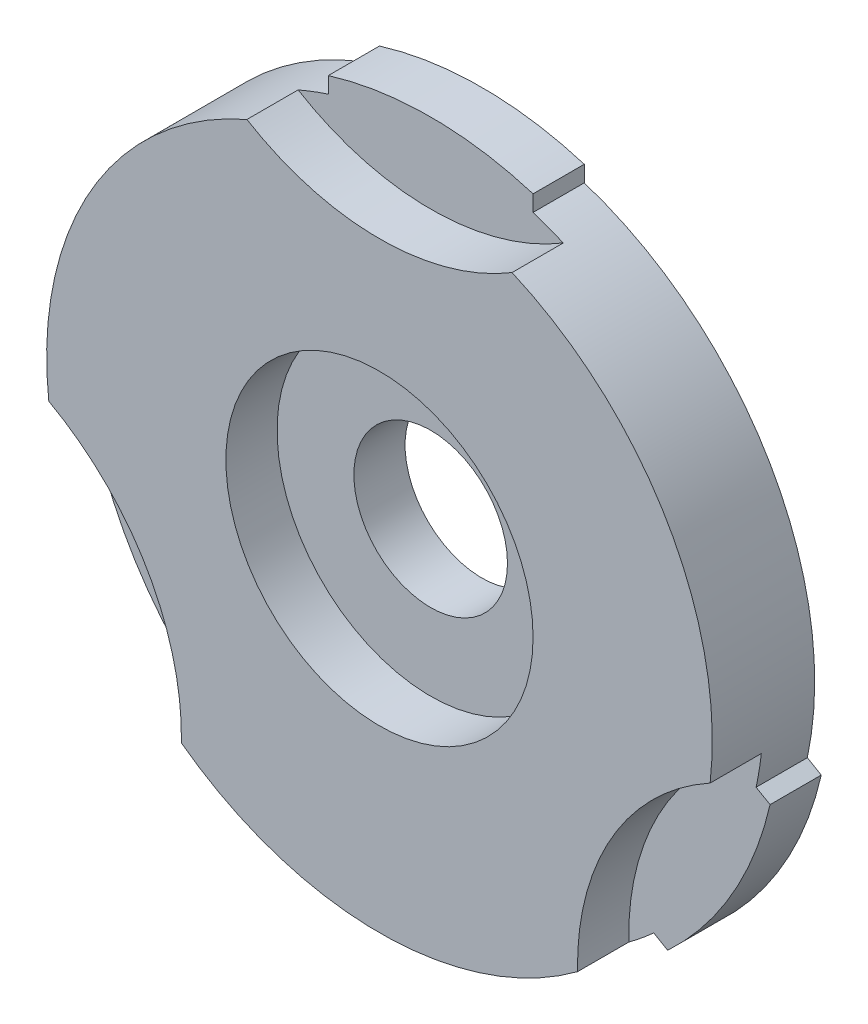
ISO-10303-21;
HEADER;
FILE_DESCRIPTION(('STEP AP214'),'2;1');
FILE_NAME('part.step','',(''),(''),'','','');
FILE_SCHEMA(('AUTOMOTIVE_DESIGN { 1 0 10303 214 1 1 1 1 }'));
ENDSEC;
DATA;
#1=APPLICATION_CONTEXT('core data for automotive mechanical design processes');
#2=APPLICATION_PROTOCOL_DEFINITION('international standard','automotive_design',2000,#1);
#3=PRODUCT_CONTEXT('',#1,'mechanical');
#4=PRODUCT('Part','Part','',(#3));
#5=PRODUCT_RELATED_PRODUCT_CATEGORY('part','',(#4));
#6=PRODUCT_DEFINITION_FORMATION('','',#4);
#7=PRODUCT_DEFINITION_CONTEXT('part definition',#1,'design');
#8=PRODUCT_DEFINITION('design','',#6,#7);
#9=PRODUCT_DEFINITION_SHAPE('','',#8);
#10=(LENGTH_UNIT() NAMED_UNIT(*) SI_UNIT(.MILLI.,.METRE.));
#11=(NAMED_UNIT(*) PLANE_ANGLE_UNIT() SI_UNIT($,.RADIAN.));
#12=(NAMED_UNIT(*) SI_UNIT($,.STERADIAN.) SOLID_ANGLE_UNIT());
#13=UNCERTAINTY_MEASURE_WITH_UNIT(LENGTH_MEASURE(1.E-05),#10,'distance_accuracy_value','');
#14=(GEOMETRIC_REPRESENTATION_CONTEXT(3) GLOBAL_UNCERTAINTY_ASSIGNED_CONTEXT((#13)) GLOBAL_UNIT_ASSIGNED_CONTEXT((#10,
#11,#12)) REPRESENTATION_CONTEXT('',''));
#15=CARTESIAN_POINT('',(0.,0.,0.));
#16=DIRECTION('',(0.,0.,1.));
#17=DIRECTION('',(1.,0.,0.));
#18=AXIS2_PLACEMENT_3D('',#15,#16,#17);
#19=CARTESIAN_POINT('',(0.,0.,10.));
#20=DIRECTION('',(0.,0.,1.));
#21=DIRECTION('',(1.,0.,0.));
#22=AXIS2_PLACEMENT_3D('',#19,#20,#21);
#23=PLANE('',#22);
#24=CARTESIAN_POINT('',(0.,102.394299444478,10.));
#25=DIRECTION('',(0.,0.,-1.));
#26=DIRECTION('',(1.,0.,0.));
#27=AXIS2_PLACEMENT_3D('',#24,#25,#26);
#28=CIRCLE('',#27,50.);
#29=CARTESIAN_POINT('',(25.8920747012508,59.6204702066735,10.));
#30=VERTEX_POINT('',#29);
#31=CARTESIAN_POINT('',(-25.8920747012508,59.6204702066735,10.));
#32=VERTEX_POINT('',#31);
#33=EDGE_CURVE('E53',#30,#32,#28,.T.);
#34=ORIENTED_EDGE('',*,*,#33,.F.);
#35=CARTESIAN_POINT('',(0.,0.,10.));
#36=DIRECTION('',(0.,0.,1.));
#37=DIRECTION('',(1.,0.,0.));
#38=AXIS2_PLACEMENT_3D('',#35,#36,#37);
#39=CIRCLE('',#38,65.);
#40=CARTESIAN_POINT('',(20.,61.8465843842649,10.));
#41=VERTEX_POINT('',#40);
#42=EDGE_CURVE('E222',#30,#41,#39,.T.);
#43=ORIENTED_EDGE('',*,*,#42,.T.);
#44=DIRECTION('',(0.,1.,0.));
#45=VECTOR('',#44,1.);
#46=CARTESIAN_POINT('',(20.,61.8465843842649,10.));
#47=LINE('',#46,#45);
#48=CARTESIAN_POINT('',(20.0000000000001,64.9923072370939,10.));
#49=VERTEX_POINT('',#48);
#50=EDGE_CURVE('E224',#41,#49,#47,.T.);
#51=ORIENTED_EDGE('',*,*,#50,.T.);
#52=CARTESIAN_POINT('',(0.,0.,10.));
#53=DIRECTION('',(0.,0.,1.));
#54=DIRECTION('',(1.,0.,0.));
#55=AXIS2_PLACEMENT_3D('',#52,#53,#54);
#56=CIRCLE('',#55,68.000000000006);
#57=CARTESIAN_POINT('',(-20.,64.9923072370939,10.));
#58=VERTEX_POINT('',#57);
#59=EDGE_CURVE('E197',#49,#58,#56,.T.);
#60=ORIENTED_EDGE('',*,*,#59,.T.);
#61=DIRECTION('',(0.,-1.,0.));
#62=VECTOR('',#61,1.);
#63=CARTESIAN_POINT('',(-20.,61.8465843842649,10.));
#64=LINE('',#63,#62);
#65=CARTESIAN_POINT('',(-20.,61.8465843842649,10.));
#66=VERTEX_POINT('',#65);
#67=EDGE_CURVE('E199',#58,#66,#64,.T.);
#68=ORIENTED_EDGE('',*,*,#67,.T.);
#69=CARTESIAN_POINT('',(0.,0.,10.));
#70=DIRECTION('',(0.,0.,1.));
#71=DIRECTION('',(1.,0.,0.));
#72=AXIS2_PLACEMENT_3D('',#69,#70,#71);
#73=CIRCLE('',#72,65.);
#74=EDGE_CURVE('E204',#66,#32,#73,.T.);
#75=ORIENTED_EDGE('',*,*,#74,.T.);
#76=EDGE_LOOP('',(#34,#43,#51,#60,#68,#75));
#77=FACE_BOUND('',#76,.T.);
#78=ADVANCED_FACE('F39',(#77),#23,.T.);
#79=CARTESIAN_POINT('',(88.6760645216287,-51.1971497222389,10.));
#80=DIRECTION('',(0.,0.,-1.));
#81=DIRECTION('',(1.,0.,0.));
#82=AXIS2_PLACEMENT_3D('',#79,#80,#81);
#83=CIRCLE('',#82,49.9999999999992);
#84=CARTESIAN_POINT('',(38.686804433928,-52.2334295513037,10.));
#85=VERTEX_POINT('',#84);
#86=CARTESIAN_POINT('',(64.5788791351778,-7.38704065537017,10.));
#87=VERTEX_POINT('',#86);
#88=EDGE_CURVE('E183',#85,#87,#83,.T.);
#89=ORIENTED_EDGE('',*,*,#88,.F.);
#90=CARTESIAN_POINT('',(0.,0.,10.));
#91=DIRECTION('',(0.,0.,1.));
#92=DIRECTION('',(1.,0.,0.));
#93=AXIS2_PLACEMENT_3D('',#90,#91,#92);
#94=CIRCLE('',#93,65.);
#95=CARTESIAN_POINT('',(43.5607132140713,-48.2438002678213,10.));
#96=VERTEX_POINT('',#95);
#97=EDGE_CURVE('E215',#85,#96,#94,.T.);
#98=ORIENTED_EDGE('',*,*,#97,.T.);
#99=DIRECTION('',(0.866025403784452,-0.499999999999977,0.));
#100=VECTOR('',#99,1.);
#101=CARTESIAN_POINT('',(43.5607132140713,-48.2438002678213,10.));
#102=LINE('',#101,#100);
#103=CARTESIAN_POINT('',(46.2849891178865,-49.8166616942358,10.));
#104=VERTEX_POINT('',#103);
#105=EDGE_CURVE('E214',#96,#104,#102,.T.);
#106=ORIENTED_EDGE('',*,*,#105,.T.);
#107=CARTESIAN_POINT('',(0.,0.,10.));
#108=DIRECTION('',(0.,0.,1.));
#109=DIRECTION('',(1.,0.,0.));
#110=AXIS2_PLACEMENT_3D('',#107,#108,#109);
#111=CIRCLE('',#110,68.000000000006);
#112=CARTESIAN_POINT('',(66.2849891178865,-15.1756455428582,10.));
#113=VERTEX_POINT('',#112);
#114=EDGE_CURVE('E220',#104,#113,#111,.T.);
#115=ORIENTED_EDGE('',*,*,#114,.T.);
#116=DIRECTION('',(-0.866025403784452,0.499999999999977,0.));
#117=VECTOR('',#116,1.);
#118=CARTESIAN_POINT('',(63.5607132140713,-13.6027841164438,10.));
#119=LINE('',#118,#117);
#120=CARTESIAN_POINT('',(63.5607132140713,-13.6027841164438,10.));
#121=VERTEX_POINT('',#120);
#122=EDGE_CURVE('E218',#113,#121,#119,.T.);
#123=ORIENTED_EDGE('',*,*,#122,.T.);
#124=EDGE_CURVE('E65',#121,#87,#39,.T.);
#125=ORIENTED_EDGE('',*,*,#124,.T.);
#126=EDGE_LOOP('',(#89,#98,#106,#115,#123,#125));
#127=FACE_BOUND('',#126,.T.);
#128=ADVANCED_FACE('F353',(#127),#23,.T.);
#129=CARTESIAN_POINT('',(-88.6760645216277,-51.1971497222418,10.));
#130=DIRECTION('',(0.,0.,-1.));
#131=DIRECTION('',(1.,0.,0.));
#132=AXIS2_PLACEMENT_3D('',#129,#130,#131);
#133=CIRCLE('',#132,50.0000000000005);
#134=CARTESIAN_POINT('',(-64.5788791351777,-7.387040655371,10.));
#135=VERTEX_POINT('',#134);
#136=CARTESIAN_POINT('',(-38.6868044339255,-52.2334295513002,10.));
#137=VERTEX_POINT('',#136);
#138=EDGE_CURVE('E296',#135,#137,#133,.T.);
#139=ORIENTED_EDGE('',*,*,#138,.F.);
#140=CARTESIAN_POINT('',(-63.5607132140714,-13.6027841164435,10.));
#141=VERTEX_POINT('',#140);
#142=EDGE_CURVE('E201',#135,#141,#73,.T.);
#143=ORIENTED_EDGE('',*,*,#142,.T.);
#144=DIRECTION('',(-0.866025403784409,-0.500000000000051,0.));
#145=VECTOR('',#144,1.);
#146=CARTESIAN_POINT('',(-63.5607132140714,-13.6027841164435,10.));
#147=LINE('',#146,#145);
#148=CARTESIAN_POINT('',(-66.2849891178866,-15.1756455428582,10.));
#149=VERTEX_POINT('',#148);
#150=EDGE_CURVE('E206',#141,#149,#147,.T.);
#151=ORIENTED_EDGE('',*,*,#150,.T.);
#152=CARTESIAN_POINT('',(0.,0.,10.));
#153=DIRECTION('',(0.,0.,1.));
#154=DIRECTION('',(1.,0.,0.));
#155=AXIS2_PLACEMENT_3D('',#152,#153,#154);
#156=CIRCLE('',#155,68.0000000000059);
#157=CARTESIAN_POINT('',(-46.2849891178866,-49.8166616942357,10.));
#158=VERTEX_POINT('',#157);
#159=EDGE_CURVE('E208',#149,#158,#156,.T.);
#160=ORIENTED_EDGE('',*,*,#159,.T.);
#161=DIRECTION('',(0.866025403784409,0.500000000000051,0.));
#162=VECTOR('',#161,1.);
#163=CARTESIAN_POINT('',(-43.5607132140715,-48.2438002678211,10.));
#164=LINE('',#163,#162);
#165=CARTESIAN_POINT('',(-43.5607132140715,-48.2438002678211,10.));
#166=VERTEX_POINT('',#165);
#167=EDGE_CURVE('E209',#158,#166,#164,.T.);
#168=ORIENTED_EDGE('',*,*,#167,.T.);
#169=EDGE_CURVE('E213',#166,#137,#94,.T.);
#170=ORIENTED_EDGE('',*,*,#169,.T.);
#171=EDGE_LOOP('',(#139,#143,#151,#160,#168,#170));
#172=FACE_BOUND('',#171,.T.);
#173=ADVANCED_FACE('F293',(#172),#23,.T.);
#174=CARTESIAN_POINT('',(0.,0.,10.));
#175=DIRECTION('',(0.,0.,-1.));
#176=DIRECTION('',(-1.,0.,0.));
#177=AXIS2_PLACEMENT_3D('',#174,#175,#176);
#178=CYLINDRICAL_SURFACE('',#177,68.000000000006);
#179=CARTESIAN_POINT('',(0.,0.,0.));
#180=DIRECTION('',(0.,0.,1.));
#181=DIRECTION('',(1.,0.,0.));
#182=AXIS2_PLACEMENT_3D('',#179,#180,#181);
#183=CIRCLE('',#182,68.000000000006);
#184=CARTESIAN_POINT('',(20.0000000000001,64.9923072370939,0.));
#185=VERTEX_POINT('',#184);
#186=CARTESIAN_POINT('',(-20.,64.9923072370939,0.));
#187=VERTEX_POINT('',#186);
#188=EDGE_CURVE('E186',#185,#187,#183,.T.);
#189=ORIENTED_EDGE('',*,*,#188,.T.);
#190=DIRECTION('',(0.,0.,-1.));
#191=VECTOR('',#190,1.);
#192=CARTESIAN_POINT('',(-20.,64.9923072370939,10.));
#193=LINE('',#192,#191);
#194=EDGE_CURVE('E11',#58,#187,#193,.T.);
#195=ORIENTED_EDGE('',*,*,#194,.F.);
#196=ORIENTED_EDGE('',*,*,#59,.F.);
#197=DIRECTION('',(0.,0.,-1.));
#198=VECTOR('',#197,1.);
#199=CARTESIAN_POINT('',(20.0000000000001,64.9923072370939,10.));
#200=LINE('',#199,#198);
#201=EDGE_CURVE('E221',#49,#185,#200,.T.);
#202=ORIENTED_EDGE('',*,*,#201,.T.);
#203=EDGE_LOOP('',(#189,#195,#196,#202));
#204=FACE_BOUND('',#203,.T.);
#205=ADVANCED_FACE('F41',(#204),#178,.T.);
#206=CARTESIAN_POINT('',(-20.,61.8465843842649,10.));
#207=DIRECTION('',(1.,0.,0.));
#208=DIRECTION('',(0.,1.,0.));
#209=AXIS2_PLACEMENT_3D('',#206,#207,#208);
#210=PLANE('',#209);
#211=DIRECTION('',(0.,-1.,0.));
#212=VECTOR('',#211,1.);
#213=CARTESIAN_POINT('',(-20.,61.8465843842649,0.));
#214=LINE('',#213,#212);
#215=CARTESIAN_POINT('',(-20.,61.8465843842649,0.));
#216=VERTEX_POINT('',#215);
#217=EDGE_CURVE('E192',#187,#216,#214,.T.);
#218=ORIENTED_EDGE('',*,*,#217,.T.);
#219=DIRECTION('',(0.,0.,-1.));
#220=VECTOR('',#219,1.);
#221=CARTESIAN_POINT('',(-20.,61.8465843842649,10.));
#222=LINE('',#221,#220);
#223=EDGE_CURVE('E50',#66,#216,#222,.T.);
#224=ORIENTED_EDGE('',*,*,#223,.F.);
#225=ORIENTED_EDGE('',*,*,#67,.F.);
#226=ORIENTED_EDGE('',*,*,#194,.T.);
#227=EDGE_LOOP('',(#218,#224,#225,#226));
#228=FACE_BOUND('',#227,.T.);
#229=ADVANCED_FACE('F345',(#228),#210,.F.);
#230=CARTESIAN_POINT('',(0.,0.,10.));
#231=DIRECTION('',(0.,0.,-1.));
#232=DIRECTION('',(-1.,0.,0.));
#233=AXIS2_PLACEMENT_3D('',#230,#231,#232);
#234=CYLINDRICAL_SURFACE('',#233,65.);
#235=CARTESIAN_POINT('',(0.,0.,0.));
#236=DIRECTION('',(0.,0.,1.));
#237=DIRECTION('',(1.,0.,0.));
#238=AXIS2_PLACEMENT_3D('',#235,#236,#237);
#239=CIRCLE('',#238,65.);
#240=CARTESIAN_POINT('',(-63.5607132140714,-13.6027841164435,0.));
#241=VERTEX_POINT('',#240);
#242=EDGE_CURVE('E230',#216,#241,#239,.T.);
#243=ORIENTED_EDGE('',*,*,#242,.T.);
#244=DIRECTION('',(0.,0.,-1.));
#245=VECTOR('',#244,1.);
#246=CARTESIAN_POINT('',(-63.5607132140714,-13.6027841164435,10.));
#247=LINE('',#246,#245);
#248=EDGE_CURVE('E275',#141,#241,#247,.T.);
#249=ORIENTED_EDGE('',*,*,#248,.F.);
#250=ORIENTED_EDGE('',*,*,#142,.F.);
#251=DIRECTION('',(0.,0.,-1.));
#252=VECTOR('',#251,1.);
#253=CARTESIAN_POINT('',(-64.5788791351743,-7.38704065537116,20.));
#254=LINE('',#253,#252);
#255=CARTESIAN_POINT('',(-64.5788791351743,-7.38704065537116,20.));
#256=VERTEX_POINT('',#255);
#257=EDGE_CURVE('E175',#256,#135,#254,.T.);
#258=ORIENTED_EDGE('',*,*,#257,.F.);
#259=CARTESIAN_POINT('',(0.,0.,20.));
#260=DIRECTION('',(0.,0.,1.));
#261=DIRECTION('',(1.,0.,0.));
#262=AXIS2_PLACEMENT_3D('',#259,#260,#261);
#263=CIRCLE('',#262,64.9999999999966);
#264=CARTESIAN_POINT('',(-25.8920747012472,59.6204702066714,20.));
#265=VERTEX_POINT('',#264);
#266=EDGE_CURVE('E163',#265,#256,#263,.T.);
#267=ORIENTED_EDGE('',*,*,#266,.F.);
#268=DIRECTION('',(0.,0.,-1.));
#269=VECTOR('',#268,1.);
#270=CARTESIAN_POINT('',(-25.8920747012472,59.6204702066714,20.));
#271=LINE('',#270,#269);
#272=EDGE_CURVE('E166',#265,#32,#271,.T.);
#273=ORIENTED_EDGE('',*,*,#272,.T.);
#274=ORIENTED_EDGE('',*,*,#74,.F.);
#275=ORIENTED_EDGE('',*,*,#223,.T.);
#276=EDGE_LOOP('',(#243,#249,#250,#258,#267,#273,#274,#275));
#277=FACE_BOUND('',#276,.T.);
#278=ADVANCED_FACE('F167',(#277),#234,.T.);
#279=CARTESIAN_POINT('',(-63.5607132140714,-13.6027841164435,10.));
#280=DIRECTION('',(0.500000000000051,-0.866025403784409,0.));
#281=DIRECTION('',(0.86602540378441,0.500000000000051,0.));
#282=AXIS2_PLACEMENT_3D('',#279,#280,#281);
#283=PLANE('',#282);
#284=DIRECTION('',(-0.866025403784409,-0.500000000000051,0.));
#285=VECTOR('',#284,1.);
#286=CARTESIAN_POINT('',(-63.5607132140714,-13.6027841164435,0.));
#287=LINE('',#286,#285);
#288=CARTESIAN_POINT('',(-66.2849891178866,-15.1756455428582,0.));
#289=VERTEX_POINT('',#288);
#290=EDGE_CURVE('E227',#241,#289,#287,.T.);
#291=ORIENTED_EDGE('',*,*,#290,.T.);
#292=DIRECTION('',(0.,0.,-1.));
#293=VECTOR('',#292,1.);
#294=CARTESIAN_POINT('',(-66.2849891178866,-15.1756455428582,10.));
#295=LINE('',#294,#293);
#296=EDGE_CURVE('E267',#149,#289,#295,.T.);
#297=ORIENTED_EDGE('',*,*,#296,.F.);
#298=ORIENTED_EDGE('',*,*,#150,.F.);
#299=ORIENTED_EDGE('',*,*,#248,.T.);
#300=EDGE_LOOP('',(#291,#297,#298,#299));
#301=FACE_BOUND('',#300,.T.);
#302=ADVANCED_FACE('F290',(#301),#283,.F.);
#303=CARTESIAN_POINT('',(0.,0.,10.));
#304=DIRECTION('',(0.,0.,-1.));
#305=DIRECTION('',(-1.,0.,0.));
#306=AXIS2_PLACEMENT_3D('',#303,#304,#305);
#307=CYLINDRICAL_SURFACE('',#306,68.0000000000059);
#308=CARTESIAN_POINT('',(0.,0.,0.));
#309=DIRECTION('',(0.,0.,1.));
#310=DIRECTION('',(1.,0.,0.));
#311=AXIS2_PLACEMENT_3D('',#308,#309,#310);
#312=CIRCLE('',#311,68.0000000000059);
#313=CARTESIAN_POINT('',(-46.2849891178866,-49.8166616942357,0.));
#314=VERTEX_POINT('',#313);
#315=EDGE_CURVE('E232',#289,#314,#312,.T.);
#316=ORIENTED_EDGE('',*,*,#315,.T.);
#317=DIRECTION('',(0.,0.,-1.));
#318=VECTOR('',#317,1.);
#319=CARTESIAN_POINT('',(-46.2849891178866,-49.8166616942357,10.));
#320=LINE('',#319,#318);
#321=EDGE_CURVE('E266',#158,#314,#320,.T.);
#322=ORIENTED_EDGE('',*,*,#321,.F.);
#323=ORIENTED_EDGE('',*,*,#159,.F.);
#324=ORIENTED_EDGE('',*,*,#296,.T.);
#325=EDGE_LOOP('',(#316,#322,#323,#324));
#326=FACE_BOUND('',#325,.T.);
#327=ADVANCED_FACE('F292',(#326),#307,.T.);
#328=CARTESIAN_POINT('',(-43.5607132140715,-48.2438002678211,10.));
#329=DIRECTION('',(-0.500000000000051,0.866025403784409,0.));
#330=DIRECTION('',(-0.866025403784409,-0.500000000000051,0.));
#331=AXIS2_PLACEMENT_3D('',#328,#329,#330);
#332=PLANE('',#331);
#333=DIRECTION('',(0.866025403784409,0.500000000000051,0.));
#334=VECTOR('',#333,1.);
#335=CARTESIAN_POINT('',(-43.5607132140715,-48.2438002678211,0.));
#336=LINE('',#335,#334);
#337=CARTESIAN_POINT('',(-43.5607132140715,-48.2438002678211,0.));
#338=VERTEX_POINT('',#337);
#339=EDGE_CURVE('E233',#314,#338,#336,.T.);
#340=ORIENTED_EDGE('',*,*,#339,.T.);
#341=DIRECTION('',(0.,0.,-1.));
#342=VECTOR('',#341,1.);
#343=CARTESIAN_POINT('',(-43.5607132140715,-48.2438002678211,10.));
#344=LINE('',#343,#342);
#345=EDGE_CURVE('E263',#166,#338,#344,.T.);
#346=ORIENTED_EDGE('',*,*,#345,.F.);
#347=ORIENTED_EDGE('',*,*,#167,.F.);
#348=ORIENTED_EDGE('',*,*,#321,.T.);
#349=EDGE_LOOP('',(#340,#346,#347,#348));
#350=FACE_BOUND('',#349,.T.);
#351=ADVANCED_FACE('F378',(#350),#332,.F.);
#352=CARTESIAN_POINT('',(0.,0.,10.));
#353=DIRECTION('',(0.,0.,-1.));
#354=DIRECTION('',(-1.,0.,0.));
#355=AXIS2_PLACEMENT_3D('',#352,#353,#354);
#356=CYLINDRICAL_SURFACE('',#355,65.);
#357=CARTESIAN_POINT('',(0.,0.,0.));
#358=DIRECTION('',(0.,0.,1.));
#359=DIRECTION('',(1.,0.,0.));
#360=AXIS2_PLACEMENT_3D('',#357,#358,#359);
#361=CIRCLE('',#360,65.);
#362=CARTESIAN_POINT('',(43.5607132140713,-48.2438002678213,0.));
#363=VERTEX_POINT('',#362);
#364=EDGE_CURVE('E231',#338,#363,#361,.T.);
#365=ORIENTED_EDGE('',*,*,#364,.T.);
#366=DIRECTION('',(0.,0.,-1.));
#367=VECTOR('',#366,1.);
#368=CARTESIAN_POINT('',(43.5607132140713,-48.2438002678213,10.));
#369=LINE('',#368,#367);
#370=EDGE_CURVE('E257',#96,#363,#369,.T.);
#371=ORIENTED_EDGE('',*,*,#370,.F.);
#372=ORIENTED_EDGE('',*,*,#97,.F.);
#373=DIRECTION('',(0.,0.,-1.));
#374=VECTOR('',#373,1.);
#375=CARTESIAN_POINT('',(38.6868044339287,-52.2334295512989,20.));
#376=LINE('',#375,#374);
#377=CARTESIAN_POINT('',(38.6868044339287,-52.2334295512989,20.));
#378=VERTEX_POINT('',#377);
#379=EDGE_CURVE('E319',#378,#85,#376,.T.);
#380=ORIENTED_EDGE('',*,*,#379,.F.);
#381=CARTESIAN_POINT('',(0.,0.,20.));
#382=DIRECTION('',(0.,0.,1.));
#383=DIRECTION('',(1.,0.,0.));
#384=AXIS2_PLACEMENT_3D('',#381,#382,#383);
#385=CIRCLE('',#384,64.9999999999966);
#386=CARTESIAN_POINT('',(-38.6868044339255,-52.2334295513002,20.));
#387=VERTEX_POINT('',#386);
#388=EDGE_CURVE('E304',#387,#378,#385,.T.);
#389=ORIENTED_EDGE('',*,*,#388,.F.);
#390=DIRECTION('',(0.,0.,-1.));
#391=VECTOR('',#390,1.);
#392=CARTESIAN_POINT('',(-38.6868044339255,-52.2334295513002,20.));
#393=LINE('',#392,#391);
#394=EDGE_CURVE('E193',#387,#137,#393,.T.);
#395=ORIENTED_EDGE('',*,*,#394,.T.);
#396=ORIENTED_EDGE('',*,*,#169,.F.);
#397=ORIENTED_EDGE('',*,*,#345,.T.);
#398=EDGE_LOOP('',(#365,#371,#372,#380,#389,#395,#396,#397));
#399=FACE_BOUND('',#398,.T.);
#400=ADVANCED_FACE('F322',(#399),#356,.T.);
#401=CARTESIAN_POINT('',(43.5607132140713,-48.2438002678213,10.));
#402=DIRECTION('',(0.499999999999977,0.866025403784452,0.));
#403=DIRECTION('',(-0.866025403784452,0.499999999999977,0.));
#404=AXIS2_PLACEMENT_3D('',#401,#402,#403);
#405=PLANE('',#404);
#406=DIRECTION('',(0.866025403784452,-0.499999999999977,0.));
#407=VECTOR('',#406,1.);
#408=CARTESIAN_POINT('',(43.5607132140713,-48.2438002678213,0.));
#409=LINE('',#408,#407);
#410=CARTESIAN_POINT('',(46.2849891178865,-49.8166616942358,0.));
#411=VERTEX_POINT('',#410);
#412=EDGE_CURVE('E240',#363,#411,#409,.T.);
#413=ORIENTED_EDGE('',*,*,#412,.T.);
#414=DIRECTION('',(0.,0.,-1.));
#415=VECTOR('',#414,1.);
#416=CARTESIAN_POINT('',(46.2849891178865,-49.8166616942358,10.));
#417=LINE('',#416,#415);
#418=EDGE_CURVE('E260',#104,#411,#417,.T.);
#419=ORIENTED_EDGE('',*,*,#418,.F.);
#420=ORIENTED_EDGE('',*,*,#105,.F.);
#421=ORIENTED_EDGE('',*,*,#370,.T.);
#422=EDGE_LOOP('',(#413,#419,#420,#421));
#423=FACE_BOUND('',#422,.T.);
#424=ADVANCED_FACE('F380',(#423),#405,.F.);
#425=CARTESIAN_POINT('',(0.,0.,10.));
#426=DIRECTION('',(0.,0.,-1.));
#427=DIRECTION('',(-1.,0.,0.));
#428=AXIS2_PLACEMENT_3D('',#425,#426,#427);
#429=CYLINDRICAL_SURFACE('',#428,68.000000000006);
#430=CARTESIAN_POINT('',(0.,0.,0.));
#431=DIRECTION('',(0.,0.,1.));
#432=DIRECTION('',(1.,0.,0.));
#433=AXIS2_PLACEMENT_3D('',#430,#431,#432);
#434=CIRCLE('',#433,68.000000000006);
#435=CARTESIAN_POINT('',(66.2849891178865,-15.1756455428582,0.));
#436=VERTEX_POINT('',#435);
#437=EDGE_CURVE('E239',#411,#436,#434,.T.);
#438=ORIENTED_EDGE('',*,*,#437,.T.);
#439=DIRECTION('',(0.,0.,-1.));
#440=VECTOR('',#439,1.);
#441=CARTESIAN_POINT('',(66.2849891178865,-15.1756455428582,10.));
#442=LINE('',#441,#440);
#443=EDGE_CURVE('E255',#113,#436,#442,.T.);
#444=ORIENTED_EDGE('',*,*,#443,.F.);
#445=ORIENTED_EDGE('',*,*,#114,.F.);
#446=ORIENTED_EDGE('',*,*,#418,.T.);
#447=EDGE_LOOP('',(#438,#444,#445,#446));
#448=FACE_BOUND('',#447,.T.);
#449=ADVANCED_FACE('F501',(#448),#429,.T.);
#450=CARTESIAN_POINT('',(63.5607132140713,-13.6027841164438,10.));
#451=DIRECTION('',(-0.499999999999977,-0.866025403784452,0.));
#452=DIRECTION('',(0.866025403784452,-0.499999999999977,0.));
#453=AXIS2_PLACEMENT_3D('',#450,#451,#452);
#454=PLANE('',#453);
#455=DIRECTION('',(-0.866025403784452,0.499999999999977,0.));
#456=VECTOR('',#455,1.);
#457=CARTESIAN_POINT('',(63.5607132140713,-13.6027841164438,0.));
#458=LINE('',#457,#456);
#459=CARTESIAN_POINT('',(63.5607132140713,-13.6027841164438,0.));
#460=VERTEX_POINT('',#459);
#461=EDGE_CURVE('E243',#436,#460,#458,.T.);
#462=ORIENTED_EDGE('',*,*,#461,.T.);
#463=DIRECTION('',(0.,0.,-1.));
#464=VECTOR('',#463,1.);
#465=CARTESIAN_POINT('',(63.5607132140713,-13.6027841164438,10.));
#466=LINE('',#465,#464);
#467=EDGE_CURVE('E253',#121,#460,#466,.T.);
#468=ORIENTED_EDGE('',*,*,#467,.F.);
#469=ORIENTED_EDGE('',*,*,#122,.F.);
#470=ORIENTED_EDGE('',*,*,#443,.T.);
#471=EDGE_LOOP('',(#462,#468,#469,#470));
#472=FACE_BOUND('',#471,.T.);
#473=ADVANCED_FACE('F387',(#472),#454,.F.);
#474=CARTESIAN_POINT('',(0.,0.,10.));
#475=DIRECTION('',(0.,0.,-1.));
#476=DIRECTION('',(-1.,0.,0.));
#477=AXIS2_PLACEMENT_3D('',#474,#475,#476);
#478=CYLINDRICAL_SURFACE('',#477,65.);
#479=CARTESIAN_POINT('',(0.,0.,0.));
#480=DIRECTION('',(0.,0.,1.));
#481=DIRECTION('',(1.,0.,0.));
#482=AXIS2_PLACEMENT_3D('',#479,#480,#481);
#483=CIRCLE('',#482,65.);
#484=CARTESIAN_POINT('',(20.,61.8465843842649,0.));
#485=VERTEX_POINT('',#484);
#486=EDGE_CURVE('E241',#460,#485,#483,.T.);
#487=ORIENTED_EDGE('',*,*,#486,.T.);
#488=DIRECTION('',(0.,0.,-1.));
#489=VECTOR('',#488,1.);
#490=CARTESIAN_POINT('',(20.,61.8465843842649,10.));
#491=LINE('',#490,#489);
#492=EDGE_CURVE('E248',#41,#485,#491,.T.);
#493=ORIENTED_EDGE('',*,*,#492,.F.);
#494=ORIENTED_EDGE('',*,*,#42,.F.);
#495=DIRECTION('',(0.,0.,-1.));
#496=VECTOR('',#495,1.);
#497=CARTESIAN_POINT('',(25.8920747012473,59.6204702066713,20.));
#498=LINE('',#497,#496);
#499=CARTESIAN_POINT('',(25.8920747012473,59.6204702066713,20.));
#500=VERTEX_POINT('',#499);
#501=EDGE_CURVE('E313',#500,#30,#498,.T.);
#502=ORIENTED_EDGE('',*,*,#501,.F.);
#503=CARTESIAN_POINT('',(0.,0.,20.));
#504=DIRECTION('',(0.,0.,1.));
#505=DIRECTION('',(1.,0.,0.));
#506=AXIS2_PLACEMENT_3D('',#503,#504,#505);
#507=CIRCLE('',#506,64.9999999999966);
#508=CARTESIAN_POINT('',(64.5788791351747,-7.38704065537195,20.));
#509=VERTEX_POINT('',#508);
#510=EDGE_CURVE('E182',#509,#500,#507,.T.);
#511=ORIENTED_EDGE('',*,*,#510,.F.);
#512=DIRECTION('',(0.,0.,-1.));
#513=VECTOR('',#512,1.);
#514=CARTESIAN_POINT('',(64.5788791351747,-7.38704065537195,20.));
#515=LINE('',#514,#513);
#516=EDGE_CURVE('E320',#509,#87,#515,.T.);
#517=ORIENTED_EDGE('',*,*,#516,.T.);
#518=ORIENTED_EDGE('',*,*,#124,.F.);
#519=ORIENTED_EDGE('',*,*,#467,.T.);
#520=EDGE_LOOP('',(#487,#493,#494,#502,#511,#517,#518,#519));
#521=FACE_BOUND('',#520,.T.);
#522=ADVANCED_FACE('F335',(#521),#478,.T.);
#523=CARTESIAN_POINT('',(20.,61.8465843842649,10.));
#524=DIRECTION('',(-1.,0.,0.));
#525=DIRECTION('',(0.,-1.,0.));
#526=AXIS2_PLACEMENT_3D('',#523,#524,#525);
#527=PLANE('',#526);
#528=DIRECTION('',(0.,1.,0.));
#529=VECTOR('',#528,1.);
#530=CARTESIAN_POINT('',(20.,61.8465843842649,0.));
#531=LINE('',#530,#529);
#532=EDGE_CURVE('E203',#485,#185,#531,.T.);
#533=ORIENTED_EDGE('',*,*,#532,.T.);
#534=ORIENTED_EDGE('',*,*,#201,.F.);
#535=ORIENTED_EDGE('',*,*,#50,.F.);
#536=ORIENTED_EDGE('',*,*,#492,.T.);
#537=EDGE_LOOP('',(#533,#534,#535,#536));
#538=FACE_BOUND('',#537,.T.);
#539=ADVANCED_FACE('F337',(#538),#527,.F.);
#540=CARTESIAN_POINT('',(0.,0.,0.));
#541=DIRECTION('',(0.,0.,1.));
#542=DIRECTION('',(1.,0.,0.));
#543=AXIS2_PLACEMENT_3D('',#540,#541,#542);
#544=PLANE('',#543);
#545=CARTESIAN_POINT('',(0.,0.,0.));
#546=DIRECTION('',(0.,0.,1.));
#547=DIRECTION('',(1.,0.,0.));
#548=AXIS2_PLACEMENT_3D('',#545,#546,#547);
#549=CIRCLE('',#548,15.);
#550=CARTESIAN_POINT('',(15.,0.,0.));
#551=VERTEX_POINT('',#550);
#552=EDGE_CURVE('E473',#551,#551,#549,.T.);
#553=ORIENTED_EDGE('',*,*,#552,.T.);
#554=EDGE_LOOP('',(#553));
#555=FACE_BOUND('',#554,.T.);
#556=ORIENTED_EDGE('',*,*,#188,.F.);
#557=ORIENTED_EDGE('',*,*,#532,.F.);
#558=ORIENTED_EDGE('',*,*,#486,.F.);
#559=ORIENTED_EDGE('',*,*,#461,.F.);
#560=ORIENTED_EDGE('',*,*,#437,.F.);
#561=ORIENTED_EDGE('',*,*,#412,.F.);
#562=ORIENTED_EDGE('',*,*,#364,.F.);
#563=ORIENTED_EDGE('',*,*,#339,.F.);
#564=ORIENTED_EDGE('',*,*,#315,.F.);
#565=ORIENTED_EDGE('',*,*,#290,.F.);
#566=ORIENTED_EDGE('',*,*,#242,.F.);
#567=ORIENTED_EDGE('',*,*,#217,.F.);
#568=EDGE_LOOP('',(#556,#557,#558,#559,#560,#561,#562,#563,#564,#565,#566,#567));
#569=FACE_BOUND('',#568,.T.);
#570=ADVANCED_FACE('F285',(#555,#569),#544,.F.);
#571=CARTESIAN_POINT('',(0.,102.394299444478,20.));
#572=DIRECTION('',(0.,0.,-1.));
#573=DIRECTION('',(-1.,0.,0.));
#574=AXIS2_PLACEMENT_3D('',#571,#572,#573);
#575=CYLINDRICAL_SURFACE('',#574,50.);
#576=ORIENTED_EDGE('',*,*,#33,.T.);
#577=ORIENTED_EDGE('',*,*,#272,.F.);
#578=CARTESIAN_POINT('',(0.,102.394299444478,20.));
#579=DIRECTION('',(0.,0.,-1.));
#580=DIRECTION('',(1.,0.,0.));
#581=AXIS2_PLACEMENT_3D('',#578,#579,#580);
#582=CIRCLE('',#581,50.);
#583=EDGE_CURVE('E177',#500,#265,#582,.T.);
#584=ORIENTED_EDGE('',*,*,#583,.F.);
#585=ORIENTED_EDGE('',*,*,#501,.T.);
#586=EDGE_LOOP('',(#576,#577,#584,#585));
#587=FACE_BOUND('',#586,.T.);
#588=ADVANCED_FACE('F190',(#587),#575,.F.);
#589=CARTESIAN_POINT('',(-88.6760645216277,-51.1971497222418,20.));
#590=DIRECTION('',(0.,0.,-1.));
#591=DIRECTION('',(-1.,0.,0.));
#592=AXIS2_PLACEMENT_3D('',#589,#590,#591);
#593=CYLINDRICAL_SURFACE('',#592,50.0000000000005);
#594=ORIENTED_EDGE('',*,*,#138,.T.);
#595=ORIENTED_EDGE('',*,*,#394,.F.);
#596=CARTESIAN_POINT('',(-88.6760645216277,-51.1971497222418,20.));
#597=DIRECTION('',(0.,0.,-1.));
#598=DIRECTION('',(1.,0.,0.));
#599=AXIS2_PLACEMENT_3D('',#596,#597,#598);
#600=CIRCLE('',#599,50.0000000000005);
#601=EDGE_CURVE('E174',#256,#387,#600,.T.);
#602=ORIENTED_EDGE('',*,*,#601,.F.);
#603=ORIENTED_EDGE('',*,*,#257,.T.);
#604=EDGE_LOOP('',(#594,#595,#602,#603));
#605=FACE_BOUND('',#604,.T.);
#606=ADVANCED_FACE('F299',(#605),#593,.F.);
#607=CARTESIAN_POINT('',(88.6760645216287,-51.1971497222389,20.));
#608=DIRECTION('',(0.,0.,-1.));
#609=DIRECTION('',(-1.,0.,0.));
#610=AXIS2_PLACEMENT_3D('',#607,#608,#609);
#611=CYLINDRICAL_SURFACE('',#610,49.9999999999992);
#612=ORIENTED_EDGE('',*,*,#88,.T.);
#613=ORIENTED_EDGE('',*,*,#516,.F.);
#614=CARTESIAN_POINT('',(88.6760645216287,-51.1971497222389,20.));
#615=DIRECTION('',(0.,0.,-1.));
#616=DIRECTION('',(1.,0.,0.));
#617=AXIS2_PLACEMENT_3D('',#614,#615,#616);
#618=CIRCLE('',#617,49.9999999999992);
#619=EDGE_CURVE('E308',#378,#509,#618,.T.);
#620=ORIENTED_EDGE('',*,*,#619,.F.);
#621=ORIENTED_EDGE('',*,*,#379,.T.);
#622=EDGE_LOOP('',(#612,#613,#620,#621));
#623=FACE_BOUND('',#622,.T.);
#624=ADVANCED_FACE('F329',(#623),#611,.F.);
#625=CARTESIAN_POINT('',(0.,51.197149722239,20.));
#626=DIRECTION('',(0.,0.,1.));
#627=DIRECTION('',(1.,0.,0.));
#628=AXIS2_PLACEMENT_3D('',#625,#626,#627);
#629=PLANE('',#628);
#630=CARTESIAN_POINT('',(0.,0.,20.));
#631=DIRECTION('',(0.,0.,1.));
#632=DIRECTION('',(1.,0.,0.));
#633=AXIS2_PLACEMENT_3D('',#630,#631,#632);
#634=CIRCLE('',#633,30.);
#635=CARTESIAN_POINT('',(30.,0.,20.));
#636=VERTEX_POINT('',#635);
#637=EDGE_CURVE('E478',#636,#636,#634,.T.);
#638=ORIENTED_EDGE('',*,*,#637,.F.);
#639=EDGE_LOOP('',(#638));
#640=FACE_BOUND('',#639,.T.);
#641=ORIENTED_EDGE('',*,*,#583,.T.);
#642=ORIENTED_EDGE('',*,*,#266,.T.);
#643=ORIENTED_EDGE('',*,*,#601,.T.);
#644=ORIENTED_EDGE('',*,*,#388,.T.);
#645=ORIENTED_EDGE('',*,*,#619,.T.);
#646=ORIENTED_EDGE('',*,*,#510,.T.);
#647=EDGE_LOOP('',(#641,#642,#643,#644,#645,#646));
#648=FACE_BOUND('',#647,.T.);
#649=ADVANCED_FACE('F179',(#640,#648),#629,.T.);
#650=CARTESIAN_POINT('',(0.,0.,10.));
#651=DIRECTION('',(0.,0.,1.));
#652=DIRECTION('',(1.,0.,0.));
#653=AXIS2_PLACEMENT_3D('',#650,#651,#652);
#654=CYLINDRICAL_SURFACE('',#653,30.);
#655=CARTESIAN_POINT('',(0.,0.,10.));
#656=DIRECTION('',(0.,0.,1.));
#657=DIRECTION('',(1.,0.,0.));
#658=AXIS2_PLACEMENT_3D('',#655,#656,#657);
#659=CIRCLE('',#658,30.);
#660=CARTESIAN_POINT('',(30.,0.,10.));
#661=VERTEX_POINT('',#660);
#662=EDGE_CURVE('E311',#661,#661,#659,.T.);
#663=ORIENTED_EDGE('',*,*,#662,.F.);
#664=EDGE_LOOP('',(#663));
#665=FACE_BOUND('',#664,.T.);
#666=ORIENTED_EDGE('',*,*,#637,.T.);
#667=EDGE_LOOP('',(#666));
#668=FACE_BOUND('',#667,.T.);
#669=ADVANCED_FACE('F414',(#665,#668),#654,.F.);
#670=CARTESIAN_POINT('',(0.,0.,10.));
#671=DIRECTION('',(0.,0.,1.));
#672=DIRECTION('',(1.,0.,0.));
#673=AXIS2_PLACEMENT_3D('',#670,#671,#672);
#674=PLANE('',#673);
#675=CARTESIAN_POINT('',(0.,0.,10.));
#676=DIRECTION('',(0.,0.,1.));
#677=DIRECTION('',(1.,0.,0.));
#678=AXIS2_PLACEMENT_3D('',#675,#676,#677);
#679=CIRCLE('',#678,15.);
#680=CARTESIAN_POINT('',(15.,0.,10.));
#681=VERTEX_POINT('',#680);
#682=EDGE_CURVE('E475',#681,#681,#679,.T.);
#683=ORIENTED_EDGE('',*,*,#682,.F.);
#684=EDGE_LOOP('',(#683));
#685=FACE_BOUND('',#684,.T.);
#686=ORIENTED_EDGE('',*,*,#662,.T.);
#687=EDGE_LOOP('',(#686));
#688=FACE_BOUND('',#687,.T.);
#689=ADVANCED_FACE('F421',(#685,#688),#674,.T.);
#690=CARTESIAN_POINT('',(0.,0.,0.));
#691=DIRECTION('',(0.,0.,1.));
#692=DIRECTION('',(1.,0.,0.));
#693=AXIS2_PLACEMENT_3D('',#690,#691,#692);
#694=CYLINDRICAL_SURFACE('',#693,15.);
#695=ORIENTED_EDGE('',*,*,#552,.F.);
#696=EDGE_LOOP('',(#695));
#697=FACE_BOUND('',#696,.T.);
#698=ORIENTED_EDGE('',*,*,#682,.T.);
#699=EDGE_LOOP('',(#698));
#700=FACE_BOUND('',#699,.T.);
#701=ADVANCED_FACE('F438',(#697,#700),#694,.F.);
#702=CLOSED_SHELL('',(#78,#128,#173,#205,#229,#278,#302,#327,#351,#400,#424,#449,#473,#522,#539,
#570,#588,#606,#624,#649,#669,#689,#701));
#703=MANIFOLD_SOLID_BREP('B2',#702);
#704=ADVANCED_BREP_SHAPE_REPRESENTATION('',(#18,#703),#14);
#705=SHAPE_DEFINITION_REPRESENTATION(#9,#704);
ENDSEC;
END-ISO-10303-21;
